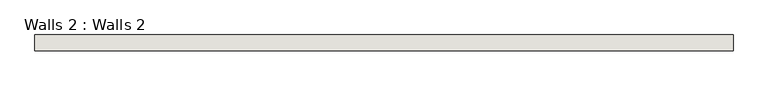
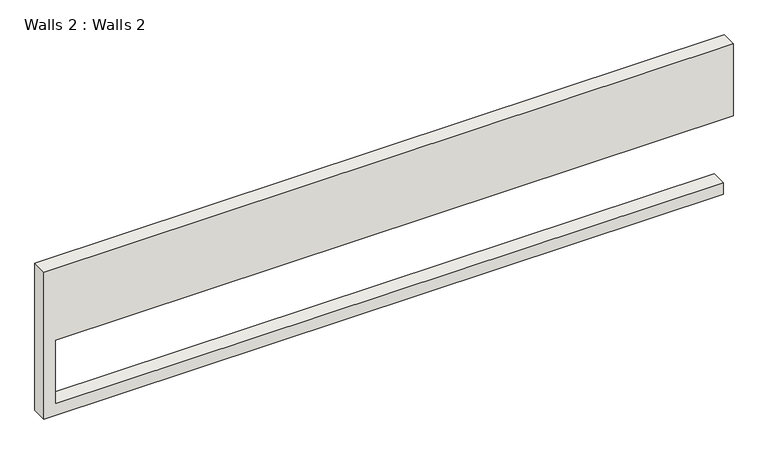
"""IFC4 building model written with IfcOpenShell, lengths in millimetres: wall geometry, Walls 2 : Walls 2."""

from ifc_helpers import new_model, si_unit, frame, origin, place, context, project, spatial, polyline, outline, extrude, source, transform, mapped, element, save


def walls_2_walls_2_ef9534d9(model_context):
    return source(origin(), model_context, "Body", "SweptSolid", [
        extrude(outline(polyline([(2649.5751957, -10580.9190315), (2649.5751957, 11835.2505118), (3048.0, 11835.2505118), (3048.0, -10207.1494882), (5264.5452246, -10207.1494882), (5264.5452246, 12159.1038637), (7776.5292316, 12159.1038637), (7776.5292316, -10580.9190315), (2649.5751957, -10580.9190315)])), frame((0.0, -9939.1578064, 0.0), z_axis=(0.0, 1.0, 0.0), x_axis=(0.0, 0.0, 1.0)), (0.0, 0.0, 1.0), 512.6837745),
    ])


if __name__ == "__main__":
    model = new_model("IFC4")
    model_context = context("Model", 3, world=origin())
    ifc_project = project(units=[si_unit("LENGTHUNIT", "METRE", prefix="MILLI")], contexts=[model_context])
    site = spatial("IfcSite", under=ifc_project)
    building = spatial("IfcBuilding", under=site)
    placement = place(None, origin())
    walls_2_walls_2_shape = walls_2_walls_2_ef9534d9(model_context)
    element("IfcWall", 1, ObjectType="Walls 2 : Walls 2", at=placement, inside=building, context=model_context, shape_type="MappedRepresentation", body=[
        mapped(walls_2_walls_2_shape, transform((0.0, 0.0, 0.0), x_axis=(1.0, 0.0, 0.0), y_axis=(0.0, 1.0, 0.0), z_axis=(0.0, 0.0, 1.0))),
    ])
    save(model, "model.ifc")

# Revit data of these elements
# Element 1 (IfcWall, "Walls 2 : Walls 2")
#   Materials on its faces: "Default Wall"
# Materials
#   "Default Wall": colour RGB 80 80 80, transparency 0
